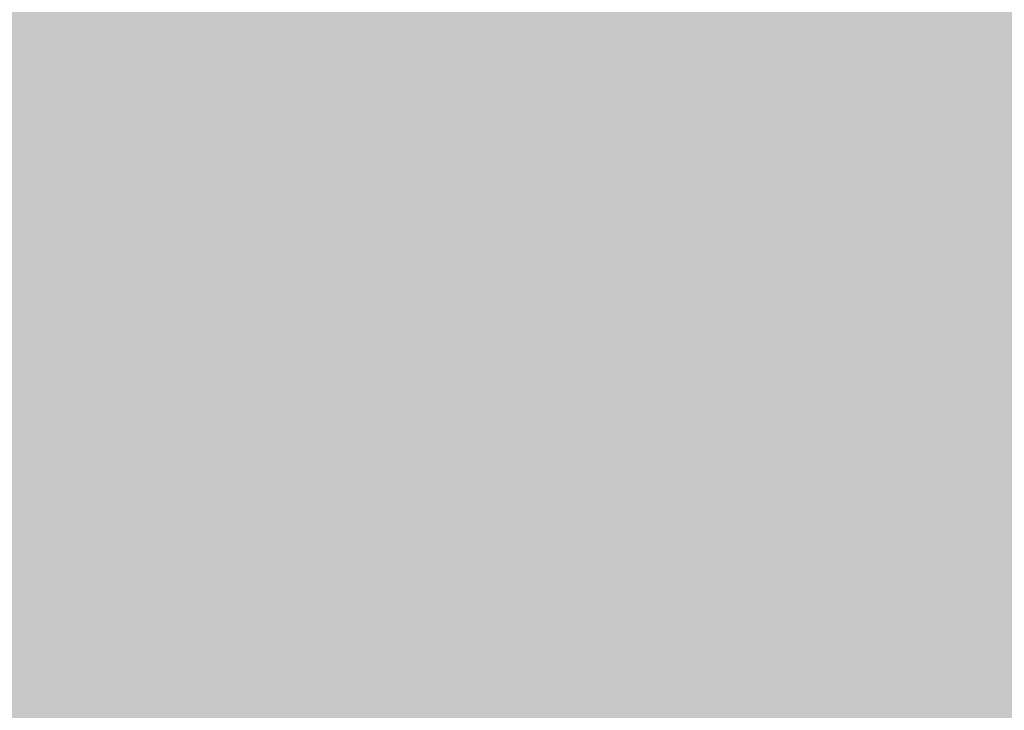
# Model space of a CAD drawing. Units: inches. Extents: x 2091 to 2899, y 967 to 2217.
# Tile 220 of 256: x 2203.2571 to 2203.4104, y 1152.3547 to 1152.4622. Entities that reach past the tile are written whole.
import ezdxf

# ---------------------------------------------------------------- set-up
doc = ezdxf.new("R2010")
doc.units = ezdxf.units.IN
doc.layers.add('A-WALL-PATT', color=141, linetype='Continuous', lineweight=13, true_color=0xadddf7)

msp = doc.modelspace()

# ---------------------------------------------------------------- hatches: boundary and pattern name
at = {"layer": 'A-WALL-PATT'}
h = msp.add_hatch(color=256, dxfattribs=at)
h.dxf.hatch_style = 1
h.paths.add_polyline_path([(2803.1436, 2050.91906), (2203.1436, 2050.91906), (2203.1436, 1090.91906), (2803.1436, 1090.91906)])
h.paths.add_polyline_path([(2635.79885, 1147.54046), (2674.52405, 1147.54046, 0.376086), (2678.52967, 1152.8802), (2678.52967, 1159.55647, 0.333335), (2674.52432, 1163.56185), (2674.52432, 1163.56185), (2674.52432, 1192.93439), (2635.80597, 1192.93439), (2597.08762, 1192.93439), (2597.08762, 1163.56185, 0.333335), (2593.08228, 1159.55647), (2593.08228, 1152.8802, 0.376086), (2597.08789, 1147.54046)], flags=0)
h.paths.add_polyline_path([(2436.01043, 1278.24078, 0.000483), (2435.95264, 1278.21503, -0.001328), (2435.93563, 1278.11169, -0.001711), (2436.11644, 1278.04076, 0.002185)], flags=0)
h.paths.add_polyline_path([(2794.1436, 1143.41906), (2794.1436, 1347.41906), (2543.37017, 1347.41906), (2543.37017, 1351.91906), (2794.1436, 1351.91906), (2794.1436, 1392.71355), (2793.9474, 1392.71355), (2793.9474, 1473.5369), (2794.1436, 1473.5369), (2794.1436, 1531.91906), (2650.1436, 1531.91906), (2650.1436, 1536.41906), (2794.1436, 1536.41906), (2794.1436, 1692.41906), (2609.37561, 1692.41906), (2609.37561, 1644.41906), (2604.87561, 1644.41906), (2604.87561, 1744.91906), (2609.37561, 1744.91906), (2609.37561, 1696.91906), (2794.1436, 1696.91906), (2794.1436, 1780.91906), (2609.6436, 1780.91906), (2493.87561, 1780.91906), (2493.87561, 1785.41906), (2609.6436, 1785.41906), (2794.1436, 1785.41906), (2794.1436, 1847.93882), (2793.95122, 1847.93882), (2793.95122, 1928.76217), (2794.1436, 1928.76217), (2794.1436, 1941.41906), (2614.1436, 1941.41906), (2614.1436, 1821.41906), (2609.6436, 1821.41906), (2609.6436, 1941.41906), (2392.1436, 1941.41906), (2392.1436, 1819.91906), (2387.6436, 1819.91906), (2387.6436, 1941.41906), (2212.1436, 1941.41906), (2212.1436, 1783.91906), (2392.1436, 1783.91906), (2392.1436, 1780.91906), (2212.1436, 1780.91906), (2212.1436, 1629.41906), (2387.6436, 1629.41906), (2387.6436, 1744.91906), (2392.1436, 1744.91906), (2392.1436, 1627.91906), (2317.1436, 1627.91906), (2317.1436, 1551.41906), (2317.1436, 1536.41906), (2459.38359, 1536.41906), (2459.38359, 1602.39648), (2463.88359, 1602.39648), (2463.88359, 1531.91906), (2456.6436, 1531.91906), (2456.6436, 1529.91906), (2452.1436, 1529.91906), (2452.1436, 1531.91906), (2312.6436, 1531.91906), (2312.6436, 1551.41906), (2306.1436, 1551.41906), (2306.1436, 1555.91906), (2308.1436, 1555.91906), (2308.1436, 1551.41906), (2312.6436, 1551.41906), (2312.6436, 1627.91906), (2212.1436, 1627.91906), (2212.1436, 1555.91906), (2270.1436, 1555.91906), (2270.1436, 1551.41906), (2212.1436, 1551.41906), (2212.1436, 1351.91906), (2272.1436, 1351.91906), (2272.1436, 1347.41906), (2212.1436, 1347.41906), (2212.1436, 1275.41906), (2308.1436, 1275.41906), (2308.1436, 1351.91906), (2452.1436, 1351.91906), (2452.1436, 1493.91906), (2456.6436, 1493.91906), (2456.6436, 1347.41906), (2312.6436, 1347.41906), (2312.6436, 1270.91906), (2212.1436, 1270.91906), (2212.1436, 1099.91906), (2281.23752, 1099.91906), (2282.87104, 1110.9138), (2282.00834, 1116.9966), (2278.55774, 1121.4204), (2268.20564, 1128.0562), (2272.08764, 1128.0562), (2273.81294, 1131.927), (2279.42034, 1134.6919), (2285.02784, 1135.2449), (2287.61584, 1137.4568), (2288.04714, 1138.0098), (2289.34114, 1140.7747), (2291.06654, 1139.6687), (2292.36054, 1135.2449), (2295.37984, 1136.9038), (2296.24254, 1135.7979), (2297.10524, 1133.033), (2300.12464, 1138.0098), (2303.14394, 1138.0098), (2304.43794, 1135.7979), (2303.14394, 1133.586), (2306.59464, 1134.6919), (2307.88874, 1133.033), (2310.90804, 1135.2449), (2313.92744, 1134.1389), (2315.62686, 1132.4271), (2308.32004, 1117.5496), (2290.20384, 1109.8079), (2288.90984, 1103.1721), (2289.27231, 1099.91906), (2434.91823, 1099.91906), (2431.59323, 1124.78806), (2429.93023, 1169.55306), (2430.92718, 1240.51969), (2435.65893, 1238.18613), (2437.13523, 1196.55406), (2438.79823, 1143.97306), (2442.67823, 1111.99806), (2446.55823, 1099.91906), (2794.1436, 1099.91906), (2794.1436, 1138.91906), (2548.03245, 1138.91906), (2548.03245, 1143.41906), (2548.03245, 1148.81906), (2546.66846, 1148.03156), (2528.68569, 1179.17862, 0.256256), (2512.03245, 1148.81906), (2512.03245, 1143.41906), (2512.03245, 1138.91906), (2507.53245, 1138.91906), (2507.53245, 1143.41906), (2507.53245, 1148.81906, 0.256256), (2490.8792, 1179.17862), (2472.89644, 1148.03156), (2471.53245, 1148.81906), (2471.53245, 1143.41906), (2467.03245, 1143.41906), (2467.03245, 1269.94579, 0.039061), (2460.90999, 1273.58006), (2467.03245, 1273.58006), (2467.03245, 1286.32536, 0.014511), (2465.21619, 1286.76191), (2467.03245, 1287.05258), (2467.03245, 1323.41906), (2471.53245, 1323.41906), (2471.53245, 1148.81906), (2489.53245, 1179.99597), (2490.89644, 1179.20847), (2490.8792, 1179.17862, -0.256256), (2507.53245, 1148.81906), (2507.53245, 1143.41906), (2512.03245, 1143.41906), (2512.03245, 1148.81906, -0.256256), (2528.68569, 1179.17862), (2528.66846, 1179.20847), (2530.03245, 1179.99597), (2548.03245, 1148.81906), (2548.03245, 1143.41906)], flags=16)
h.paths.add_polyline_path([(2607.76855, 1200.94508), (2607.76855, 1265.03063), (2597.08762, 1281.05201), (2619.78459, 1281.05201), (2627.79528, 1337.12686), (2635.79885, 1337.12686), (2643.81666, 1337.12686), (2651.82736, 1281.05201), (2674.52432, 1281.05201), (2663.8434, 1265.03063), (2663.8434, 1200.94508), (2635.80597, 1200.94508)], flags=0)
edge = h.paths.add_edge_path(flags=0)
edge.add_ellipse((13303.89622, 1272.99872), major_axis=(-10595.31304, 0), ratio=0.84230387009, start_angle=0.628237219, end_angle=0.6465541, ccw=False)
edge.add_ellipse((2711.70045, 1156.85268), major_axis=(2.21977, 0), ratio=0.8423039, start_angle=111.53524, end_angle=180.62824, ccw=False)
edge.add_ellipse((13303.15629, 1272.99872), major_axis=(-10593.02631, 0), ratio=0.84230386954, start_angle=0.528271472, end_angle=0.646554097, ccw=False)
edge.add_line((2710.7646, 1175.3333), (2710.12999, 1175.3333))
edge.add_ellipse((2710.12999, 1176.57978), major_axis=(1.47985, 0), ratio=0.8423039, start_angle=180, end_angle=270, ccw=False)
edge.add_line((2708.65014, 1176.57978), (2708.65014, 1200.78291))
edge.add_ellipse((2710.12999, 1200.78291), major_axis=(1.47985, 0), ratio=0.8423039, start_angle=90, end_angle=180, ccw=False)
edge.add_line((2710.12999, 1202.02939), (2710.46508, 1202.02939))
edge.add_ellipse((13303.15629, 1272.99872), major_axis=(-10593.02631, 0), ratio=0.84230386954, start_angle=-0.090229089, end_angle=0.383866779, ccw=False)
edge.add_ellipse((2710.12999, 1290.92703), major_axis=(-1.47985, 0), ratio=0.8423039, start_angle=0, end_angle=90, ccw=False)
edge.add_line((2708.65014, 1290.92703), (2708.65014, 1315.13017))
edge.add_ellipse((2710.12999, 1315.13017), major_axis=(-1.47985, 0), ratio=0.8423039, start_angle=-90, end_angle=0, ccw=False)
edge.add_line((2710.12999, 1316.37665), (2710.70631, 1316.37665))
edge.add_ellipse((3238.40172, 1296.28957), major_axis=(528.234, 0), ratio=0.84230387, start_angle=176.3495724, end_angle=177.8200497, ccw=False)
edge.add_ellipse((2775.06304, 1071.4507), major_axis=(313.30776, 0), ratio=0.84230387, start_angle=102.1259656, end_angle=103.780529, ccw=False)
edge.add_ellipse((2775.06304, 1078.3057), major_axis=(-305.30289, 0), ratio=0.84230387, start_angle=-79.790461, end_angle=-77.5553727, ccw=False)
edge.add_ellipse((2695.14177, 1541.97538), major_axis=(-250.96022, 0), ratio=0.84230387, start_angle=99.256566, end_angle=102.5549326)
edge.add_line((2741.41033, 1334.21426), (2747.13255, 1337.37848))
edge.add_ellipse((2747.53862, 1336.85748), major_axis=(-0.73992, 0), ratio=0.842304, start_angle=270, end_angle=307.93313, ccw=False)
edge.add_ellipse((2747.53862, 1336.85748), major_axis=(-0.73992, 0), ratio=0.842304, start_angle=232.06687, end_angle=270, ccw=False)
edge.add_line((2747.94469, 1337.37848), (2753.66691, 1334.21426))
edge.add_ellipse((2799.93547, 1541.97538), major_axis=(250.96022, 0), ratio=0.84230387, start_angle=257.4450674, end_angle=260.743434)
edge.add_ellipse((2720.01419, 1078.3057), major_axis=(305.30289, 0), ratio=0.84230387, start_angle=77.5553727, end_angle=79.790461, ccw=False)
edge.add_ellipse((2720.01419, 1071.4507), major_axis=(-313.30776, 0), ratio=0.84230387, start_angle=256.219471, end_angle=257.8740344, ccw=False)
edge.add_ellipse((2256.67551, 1296.28957), major_axis=(-528.234, 0), ratio=0.84230387, start_angle=182.1799503, end_angle=183.6504276, ccw=False)
edge.add_line((2784.37092, 1316.37665), (2784.94725, 1316.37665))
edge.add_ellipse((2784.94725, 1315.13017), major_axis=(1.47985, 0), ratio=0.8423039, start_angle=0, end_angle=90, ccw=False)
edge.add_line((2786.42709, 1315.13017), (2786.42709, 1290.92703))
edge.add_ellipse((2784.94725, 1290.92703), major_axis=(1.47985, 0), ratio=0.8423039, start_angle=270, end_angle=360, ccw=False)
edge.add_ellipse((-7808.07906, 1272.99872), major_axis=(10593.02631, 0), ratio=0.84230386954, start_angle=-0.383866779, end_angle=0.090229089, ccw=False)
edge.add_line((2784.61216, 1202.02939), (2784.94725, 1202.02939))
edge.add_ellipse((2784.94725, 1200.78291), major_axis=(1.47985, 0), ratio=0.8423039, start_angle=0, end_angle=90, ccw=False)
edge.add_line((2786.42709, 1200.78291), (2786.42709, 1176.57978))
edge.add_ellipse((2784.94725, 1176.57978), major_axis=(-1.47985, 0), ratio=0.8423039, start_angle=90, end_angle=180, ccw=False)
edge.add_line((2784.94725, 1175.3333), (2784.31264, 1175.3333))
edge.add_ellipse((-7808.07906, 1272.99872), major_axis=(10593.02631, 0), ratio=0.84230386954, start_angle=-0.618643196, end_angle=-0.528271472, ccw=False)
edge.add_ellipse((2783.37678, 1156.85268), major_axis=(-2.21977, 0), ratio=0.8423039, start_angle=179.37176, end_angle=248.46476, ccw=False)
edge.add_ellipse((-7808.81898, 1272.99872), major_axis=(-10595.31304, 0), ratio=0.84230386576, start_angle=179.353445923, end_angle=179.371762803, ccw=False)
edge.add_ellipse((2780.2973, 1153.50079), major_axis=(-5.24643, 0), ratio=0.8423039, start_angle=90, end_angle=179.35345, ccw=False)
edge.add_line((2780.2973, 1149.08171), (2714.77993, 1149.08171))
edge.add_ellipse((2714.77993, 1153.50079), major_axis=(5.24643, 0), ratio=0.8423039, start_angle=180.64655, end_angle=270, ccw=False)
edge = h.paths.add_edge_path(flags=0)
edge.add_line((2718.18737, 1151.00783), (2718.18737, 1170.47236))
edge.add_ellipse((2721.14706, 1170.47236), major_axis=(-2.95969, 0), ratio=0.8423039, start_angle=-90, end_angle=0, ccw=False)
edge.add_line((2721.14706, 1172.96532), (2773.93017, 1172.96532))
edge.add_ellipse((2773.93017, 1170.47236), major_axis=(-2.95969, 0), ratio=0.8423039, start_angle=180, end_angle=270, ccw=False)
edge.add_line((2776.88987, 1170.47236), (2776.88987, 1151.00783))
edge.add_line((2776.88987, 1151.00783), (2718.18737, 1151.00783))
edge = h.paths.add_edge_path(flags=0)
edge.add_line((2718.18737, 1180.23415), (2718.18737, 1199.05783))
edge.add_ellipse((2747.53862, 1320.39864), major_axis=(147.01792, 0), ratio=0.84230387, start_angle=256.4018653, end_angle=283.5981347)
edge.add_line((2776.88987, 1199.05783), (2776.88987, 1180.23415))
edge.add_ellipse((2747.53862, 1301.57496), major_axis=(147.01792, 0), ratio=0.84230387, start_angle=256.4018653, end_angle=283.5981347, ccw=False)
edge = h.paths.add_edge_path(flags=0)
edge.add_ellipse((13303.15629, 1272.99872), major_axis=(-10591.54646, 0), ratio=0.84230386955, start_angle=0.055594314, end_angle=0.377764194, ccw=False)
edge.add_line((2711.61686, 1262.72171), (2715.66741, 1249.4954))
edge.add_ellipse((6413.89196, 1241.69192), major_axis=(-3698.23616, 0), ratio=0.8423038695, start_angle=-0.12089737, end_angle=0.36407635)
edge.add_line((2715.76104, 1218.19245), (2711.93431, 1203.16736))
edge = h.paths.add_edge_path(flags=0)
edge.add_line((2718.18737, 1251.07457), (2716.00249, 1267.45044))
edge.add_ellipse((2742.15117, 1202.18954), major_axis=(81.77258, 0), ratio=0.84230387, start_angle=94.277421, end_angle=111.8349538, ccw=False)
edge.add_line((2737.00975, 1270.93063), (2758.06748, 1270.93063))
edge.add_ellipse((2752.92606, 1202.18954), major_axis=(81.77258, 0), ratio=0.84230387, start_angle=68.1650462, end_angle=85.722579, ccw=False)
edge.add_line((2779.07475, 1267.45044), (2776.88987, 1251.07457))
edge.add_ellipse((2750.33806, 1187.88536), major_axis=(79.57966, 0), ratio=0.84230387, start_angle=67.2080851, end_angle=85.1299304)
edge.add_line((2756.03466, 1254.74366), (2739.04258, 1254.74366))
edge.add_ellipse((2744.73917, 1187.88536), major_axis=(79.57966, 0), ratio=0.84230387, start_angle=94.8700696, end_angle=112.7919149)
edge = h.paths.add_edge_path(flags=0)
edge.add_line((2783.14293, 1203.16736), (2779.31619, 1218.19245))
edge.add_ellipse((-918.81473, 1241.69192), major_axis=(3698.23616, 0), ratio=0.8423038695, start_angle=-0.36407635, end_angle=0.12089737)
edge.add_line((2779.40983, 1249.4954), (2783.46037, 1262.72171))
edge.add_ellipse((-7808.07906, 1272.99872), major_axis=(-10591.54646, 0), ratio=0.84230386954, start_angle=179.622235806, end_angle=179.944405687, ccw=False)
edge = h.paths.add_edge_path(flags=0)
edge.add_ellipse((2734.20089, 1286.69044), major_axis=(-0.35661, 6.34008), ratio=0.6038336, start_angle=89.002014, end_angle=253.657408, ccw=False)
edge.add_line((2730.369, 1286.54181), (2730.369, 1301.35198))
edge.add_line((2730.369, 1301.35198), (2735.91331, 1305.2148))
edge.add_ellipse((2736.38492, 1304.73456), major_axis=(0.73992, 0), ratio=0.842304, start_angle=90, end_angle=134.48021, ccw=False)
edge.add_line((2736.38492, 1305.3578), (2738.03278, 1305.3578))
edge.add_line((2738.03278, 1305.3578), (2738.03278, 1307.70793))
edge.add_ellipse((2794.20164, 1307.70793), major_axis=(56.16886, 0), ratio=0.84230387, start_angle=150.56143, end_angle=180, ccw=False)
edge.add_ellipse((2700.87559, 1307.70793), major_axis=(-56.16886, 0), ratio=0.84230387, start_angle=180, end_angle=209.43857, ccw=False)
edge.add_line((2757.04445, 1307.70793), (2757.04445, 1305.3578))
edge.add_line((2757.04445, 1305.3578), (2758.69232, 1305.3578))
edge.add_ellipse((2758.69232, 1304.73456), major_axis=(-0.73992, 0), ratio=0.842304, start_angle=225.51979, end_angle=270, ccw=False)
edge.add_line((2759.16392, 1305.2148), (2764.70823, 1301.35198))
edge.add_line((2764.70823, 1301.35198), (2764.70823, 1286.54181))
edge.add_ellipse((2760.87634, 1286.69044), major_axis=(0.35661, 6.34008), ratio=0.6038336, start_angle=106.342592, end_angle=270.997986, ccw=False)
edge.add_line((2757.04445, 1285.79709), (2757.04445, 1307.70793))
edge.add_ellipse((2700.87559, 1307.70793), major_axis=(-56.16886, 0), ratio=0.84230387, start_angle=180, end_angle=209.43857)
edge.add_ellipse((2794.20164, 1307.70793), major_axis=(56.16886, 0), ratio=0.84230387, start_angle=150.56143, end_angle=180)
edge.add_line((2738.03278, 1307.70793), (2738.03278, 1285.79709))
h.paths.add_polyline_path([(2417.81227, 1104.4497), (2413.49227, 1102.5297), (2410.61227, 1103.9697), (2409.17227, 1106.3697), (2407.25227, 1107.3297), (2406.29227, 1109.7297), (2405.33227, 1114.0497), (2405.33227, 1117.8897), (2406.29227, 1120.1297), (2407.25227, 1119.8097), (2408.84832, 1118.32766), (2410.17395, 1119.42417), (2410.21127, 1120.4057), (2411.04073, 1121.41905), (2410.69927, 1119.8587), (2410.17395, 1119.42417), (2410.08845, 1117.17611), (2411.13284, 1116.20632), (2413.97227, 1119.3297), (2416.85227, 1120.7697), (2416.86972, 1120.79878), (2417.03507, 1119.40512), (2417.89621, 1118.14338), (2418.29227, 1118.3697), (2419.54445, 1120.03927), (2419.36092, 1118.38749), (2419.03211, 1119.35615), (2418.39894, 1118.51193), (2419.25227, 1114.5297), (2418.79409, 1107.19879)], flags=0)
h.paths.add_polyline_path([(2508.87017, 1347.41906), (2508.37017, 1347.41906), (2508.37017, 1351.91906), (2508.87017, 1351.91906)], flags=0)
h.paths.add_polyline_path([(2473.37017, 1347.41906), (2472.37017, 1347.41906), (2467.87017, 1347.41906), (2467.87017, 1455.41906), (2472.37017, 1455.41906), (2472.37017, 1352.41906), (2473.37017, 1352.41906)], flags=0)
h.paths.add_polyline_path([(2352.10624, 1217.4462), (2349.22624, 1218.8862), (2347.78624, 1221.2862), (2345.86624, 1222.2462), (2344.90624, 1224.6462), (2343.94624, 1228.9662), (2343.94624, 1232.8062), (2344.90624, 1235.0462), (2345.86624, 1234.7262), (2347.46229, 1233.24415), (2348.78792, 1234.34066), (2348.82524, 1235.3222), (2349.6547, 1236.33555), (2349.31324, 1234.7752), (2348.78792, 1234.34066), (2348.70242, 1232.0926), (2349.74681, 1231.12282), (2352.58624, 1234.2462), (2355.46624, 1235.6862), (2355.48369, 1235.71528), (2355.64904, 1234.32161), (2356.51018, 1233.05988), (2356.90624, 1233.2862), (2358.15842, 1234.95576), (2357.97489, 1233.30398), (2357.64608, 1234.27264), (2357.01291, 1233.42842), (2357.86624, 1229.4462), (2357.40806, 1222.11529), (2356.42624, 1219.3662)], flags=0)
h.paths.add_polyline_path([(2348.2968, 1112.22442), (2347.0138, 1112.31042), (2345.5298, 1114.12742), (2345.7318, 1115.85842), (2346.8118, 1116.98242), (2346.8118, 1114.64642), (2345.8668, 1114.21442), (2346.8798, 1114.30042)], flags=0)
h.paths.add_polyline_path([(2347.0138, 1110.92642), (2346.2718, 1110.49342), (2346.6098, 1111.18642)], flags=0)
h.paths.add_polyline_path([(2345.8668, 1118.19442), (2345.5298, 1117.32942), (2343.7078, 1118.02142), (2344.3828, 1118.62642)], flags=0)
h.paths.add_polyline_path([(2346.6768, 1109.28242), (2346.0698, 1108.07142), (2345.8668, 1110.06142)], flags=0)
h.paths.add_polyline_path([(2345.0568, 1119.75142), (2343.6398, 1119.75142), (2343.9778, 1121.13542)], flags=0)
h.paths.add_polyline_path([(2345.2598, 1116.55042), (2345.1248, 1115.85842), (2344.9218, 1115.68542), (2344.7198, 1116.37742)], flags=0)
h.paths.add_polyline_path([(2345.6648, 1112.31042), (2345.4618, 1111.53242), (2344.0448, 1111.96442), (2344.6518, 1112.57042)], flags=0)
h.paths.add_polyline_path([(2345.1918, 1113.34942), (2344.4498, 1113.86842), (2344.7198, 1114.38742)], flags=0)
h.paths.add_polyline_path([(2344.6518, 1116.80942), (2344.1798, 1115.68542), (2344.6518, 1115.33942), (2343.9098, 1114.90642), (2343.0328, 1115.94442), (2343.6398, 1116.46342)], flags=0)
h.paths.add_polyline_path([(2345.8668, 1106.68642), (2344.9898, 1105.56242), (2344.5168, 1106.60042)], flags=0)
h.paths.add_polyline_path([(2344.8548, 1110.06142), (2344.5168, 1109.28242), (2344.1128, 1109.71542)], flags=0)
h.paths.add_polyline_path([(2344.0448, 1113.52242), (2343.4378, 1113.08942), (2342.7628, 1113.95442)], flags=0)
h.paths.add_polyline_path([(2344.3148, 1111.01242), (2342.9648, 1110.32042), (2342.9648, 1111.09942)], flags=0)
h.paths.add_polyline_path([(2345.1248, 1104.69742), (2344.5848, 1103.74542), (2344.4498, 1104.26442)], flags=0)
h.paths.add_polyline_path([(2342.8298, 1121.22242), (2341.7498, 1120.53042), (2340.5358, 1121.04942), (2340.1308, 1121.82842), (2340.6708, 1122.95242), (2341.1428, 1121.82842), (2341.6148, 1122.00142)], flags=0)
h.paths.add_polyline_path([(2342.9648, 1119.75142), (2343.0328, 1118.45342), (2342.0878, 1118.02142), (2342.0198, 1119.49142)], flags=0)
h.paths.add_polyline_path([(2342.6948, 1116.89642), (2341.9528, 1116.63642), (2342.0198, 1117.32942)], flags=0)
h.paths.add_polyline_path([(2343.0328, 1112.22442), (2342.0198, 1111.79142), (2341.5478, 1112.22442), (2342.3578, 1113.34942)], flags=0)
h.paths.add_polyline_path([(2343.7748, 1104.43742), (2342.6278, 1102.88042), (2342.6948, 1104.61042), (2343.4378, 1105.12942)], flags=0)
h.paths.add_polyline_path([(2342.0198, 1115.07942), (2340.8058, 1115.51242), (2340.9408, 1116.37742)], flags=0)
h.paths.add_polyline_path([(2341.4808, 1120.09742), (2341.4808, 1119.40542), (2341.0758, 1119.57842), (2341.1428, 1120.09742)], flags=0)
h.paths.add_polyline_path([(2341.8178, 1114.47342), (2340.9408, 1113.08942), (2340.8058, 1114.56042)], flags=0)
h.paths.add_polyline_path([(2341.1428, 1118.54042), (2340.9408, 1116.98242), (2339.0508, 1117.67542), (2339.0508, 1118.62642)], flags=0)
h.paths.add_polyline_path([(2342.6948, 1101.66842), (2341.9528, 1101.84142), (2342.5598, 1102.36142)], flags=0)
h.paths.add_polyline_path([(2340.3328, 1119.66542), (2338.4438, 1119.57842), (2337.9038, 1120.35742), (2339.6578, 1120.61642)], flags=0)
h.paths.add_polyline_path([(2340.3328, 1115.33942), (2340.0628, 1113.69542), (2339.3878, 1115.33942)], flags=0)
h.paths.add_polyline_path([(2341.8178, 1103.83142), (2341.5478, 1102.88042), (2341.1428, 1103.65842)], flags=0)
h.paths.add_polyline_path([(2339.0508, 1122.86642), (2337.2958, 1121.82842), (2337.0938, 1123.12542), (2337.7688, 1123.81842)], flags=0)
h.paths.add_polyline_path([(2339.1178, 1121.74142), (2338.8478, 1121.22242), (2338.1738, 1121.04942), (2338.3758, 1121.56842)], flags=0)
h.paths.add_polyline_path([(2339.1858, 1119.31942), (2338.6458, 1118.71342), (2338.2408, 1118.10742), (2338.2408, 1118.88642)], flags=0)
h.paths.add_polyline_path([(2341.1428, 1101.92842), (2340.6028, 1101.23642), (2340.0628, 1101.84142), (2340.6028, 1102.36142)], flags=0)
h.paths.add_polyline_path([(2337.6338, 1117.76142), (2336.6208, 1118.28042), (2337.2958, 1118.97242)], flags=0)
h.paths.add_polyline_path([(2336.8238, 1119.57842), (2334.7988, 1118.97242), (2335.2038, 1120.35742), (2336.5538, 1120.87642)], flags=0)
h.paths.add_polyline_path([(2339.1178, 1100.45742), (2337.3638, 1100.54342), (2336.7558, 1101.23642)], flags=0)
h.paths.add_polyline_path([(2336.3508, 1122.43342), (2336.0138, 1121.91442), (2334.9338, 1122.43342), (2334.5288, 1123.47142), (2335.7438, 1122.77942)], flags=0)
h.paths.add_polyline_path([(2334.7318, 1120.87642), (2334.2588, 1120.35742), (2334.0568, 1120.78942), (2334.5968, 1121.30842)], flags=0)
h.paths.add_polyline_path([(2334.4618, 1122.17442), (2332.5718, 1121.30842), (2331.3568, 1122.17442), (2332.0998, 1122.86642)], flags=0)
h.paths.add_polyline_path([(2334.2588, 1118.54042), (2333.3818, 1118.45342), (2333.6518, 1119.31942)], flags=0)
h.paths.add_polyline_path([(2335.5418, 1102.27442), (2334.1918, 1102.62042), (2335.2718, 1103.31242)], flags=0)
h.paths.add_polyline_path([(2332.7068, 1119.66542), (2331.6948, 1120.44342), (2332.5048, 1120.78942)], flags=0)
h.paths.add_polyline_path([(2334.7318, 1101.14942), (2333.5168, 1101.58242), (2333.9888, 1101.75542)], flags=0)
h.paths.add_polyline_path([(2332.6398, 1116.63642), (2331.0868, 1116.29042), (2331.9648, 1118.19442)], flags=0)
h.paths.add_polyline_path([(2330.7498, 1121.56842), (2330.2768, 1120.27042), (2328.5228, 1119.31942), (2328.9948, 1121.04942)], flags=0)
h.paths.add_polyline_path([(2330.7498, 1118.62642), (2330.0078, 1117.50242), (2329.8728, 1118.02142)], flags=0)
h.paths.add_polyline_path([(2332.0998, 1102.36142), (2330.5468, 1102.01442), (2331.6948, 1102.96642)], flags=0)
h.paths.add_polyline_path([(2329.5348, 1113.60842), (2329.0628, 1112.31042), (2328.5898, 1113.34942)], flags=0)
h.paths.add_polyline_path([(2328.3878, 1117.84842), (2327.5098, 1116.55042), (2327.1728, 1117.76142)], flags=0)
h.paths.add_polyline_path([(2329.7378, 1106.51342), (2329.5348, 1105.30242), (2328.2528, 1106.08142)], flags=0)
h.paths.add_polyline_path([(2328.6578, 1114.38742), (2328.0498, 1114.12742), (2328.3198, 1114.90642)], flags=0)
h.paths.add_polyline_path([(2328.3198, 1112.22442), (2327.1058, 1112.13742), (2326.7008, 1112.65642)], flags=0)
h.paths.add_polyline_path([(2326.9028, 1115.25242), (2326.7008, 1114.12742), (2325.2158, 1113.60842), (2326.0928, 1115.33942)], flags=0)
h.paths.add_polyline_path([(2326.6328, 1108.33042), (2326.0928, 1107.37942), (2325.8908, 1108.50342), (2326.4978, 1109.10942)], flags=0)
h.paths.add_polyline_path([(2615.1436, 1531.91906), (2609.6436, 1531.91906), (2609.6436, 1620.41906), (2614.1436, 1620.41906), (2614.1436, 1536.41906), (2615.1436, 1536.41906)], flags=0)
h.paths.add_polyline_path([(2545.1436, 1563.41906), (2464.1436, 1563.41906), (2464.1436, 1632.41906), (2509.1436, 1632.41906), (2509.1436, 1627.91906), (2509.1436, 1603.91906), (2468.6436, 1603.91906), (2468.6436, 1567.91906), (2540.6436, 1567.91906), (2540.6436, 1591.91906), (2545.1436, 1591.91906)], flags=0)
h.paths.add_polyline_path([(2388.96905, 1549.98573), (2357.43418, 1549.98573), (2357.43418, 1623.36078), (2399.36278, 1623.36078), (2435.68947, 1623.36078), (2435.59255, 1602.55927), (2435.59255, 1602.39648), (2388.96905, 1602.39648)], flags=0)
h.paths.add_polyline_path([(2388.88063, 1555.80915), (2374.90443, 1555.80915), (2374.90443, 1600.57156), (2374.90443, 1615.45765), (2406.35088, 1615.45765), (2406.35088, 1618.93943), (2412.17429, 1615.45765), (2406.35088, 1611.97586), (2406.35088, 1615.45765), (2388.88063, 1615.45765)], flags=0)
h.paths.add_polyline_path([(2568.87561, 1644.41906), (2453.37561, 1644.41906), (2453.37561, 1785.41906), (2457.87561, 1785.41906), (2457.87561, 1648.91906), (2568.87561, 1648.91906)], flags=0)
h.paths.add_polyline_path([(2212.1436, 1945.91906), (2212.1436, 2041.91906), (2794.1436, 2041.91906), (2794.1436, 1945.91906)], flags=16)
h.paths.add_polyline_path([(2271.08273, 1964.31724), (2776.85297, 1964.31724), (2776.85297, 2037.16962), (2271.08273, 2037.16962)], flags=8)
h.paths.add_polyline_path([(2380.64929, 1536.82414), (2461.04081, 1536.82414), (2461.04081, 1554.65259), (2380.64929, 1554.65259)], flags=8)
h.paths.add_polyline_path([(2240.75571, 1609.72545), (2309.18583, 1609.72545), (2309.18583, 1617.6982), (2240.75571, 1617.6982)], flags=8)
h.paths.add_polyline_path([(2212.67726, 1313.5041), (2282.59152, 1313.5041), (2282.59152, 1322.74524), (2212.67726, 1322.74524)], flags=8)
h.paths.add_polyline_path([(2457.11198, 1114.77857), (2558.48158, 1114.77857), (2558.48158, 1142.21968), (2457.11198, 1142.21968)], flags=8)
h.paths.add_polyline_path([(2473.44234, 1273.01007), (2604.64123, 1273.01007), (2604.64123, 1318.34693), (2473.44234, 1318.34693)], flags=8)
h.paths.add_polyline_path([(2638.8763, 1626.97743), (2684.25037, 1627.97674), (2684.03848, 1637.59749), (2638.66442, 1636.59819)], flags=8)
h.paths.add_polyline_path([(2537.59055, 1453.79345), (2628.38955, 1453.79345), (2628.38955, 1475.34481), (2537.59055, 1475.34481)], flags=8)
h.paths.add_polyline_path([(2504.13764, 1714.6324), (2554.64719, 1714.6324), (2554.64719, 1730.23771), (2504.13764, 1730.23771)], flags=8)
h.paths.add_polyline_path([(2487.50118, 1575.65187), (2535.09712, 1575.65187), (2535.09712, 1598.37765), (2487.50118, 1598.37765)], flags=8)
h.paths.add_polyline_path([(2709.0994, 1735.71028), (2740.0166, 1735.71028), (2740.0166, 1749.93764), (2709.0994, 1749.93764)], flags=8)
h.paths.add_polyline_path([(2442.43842, 1792.17166), (2564.72884, 1792.17166), (2564.72884, 1842.00016), (2442.43842, 1842.00016)], flags=8)
h.paths.add_polyline_path([(2655.8158, 1809.64408), (2789.52014, 1806.6938), (2790.08498, 1832.29164), (2656.38064, 1835.24192)], flags=8)
h.paths.add_polyline_path([(2234.8427, 1797.72014), (2368.59285, 1794.76885), (2369.16072, 1820.50413), (2235.41056, 1823.45542)], flags=8)
h.paths.add_polyline_path([(2245.13847, 1644.00633), (2398.42773, 1640.6239), (2398.99484, 1666.32482), (2245.70557, 1669.70725)], flags=8)
h.paths.add_polyline_path([(2306.14285, 1431.16852), (2413.76831, 1428.79369), (2414.33315, 1454.39153), (2306.70768, 1456.76636)], flags=8)
h.paths.add_polyline_path([(2306.83458, 1458.23314), (2393.38048, 1456.32345), (2393.93281, 1481.35436), (2307.38691, 1483.26405)], flags=8)

doc.saveas('drawing.dxf')
